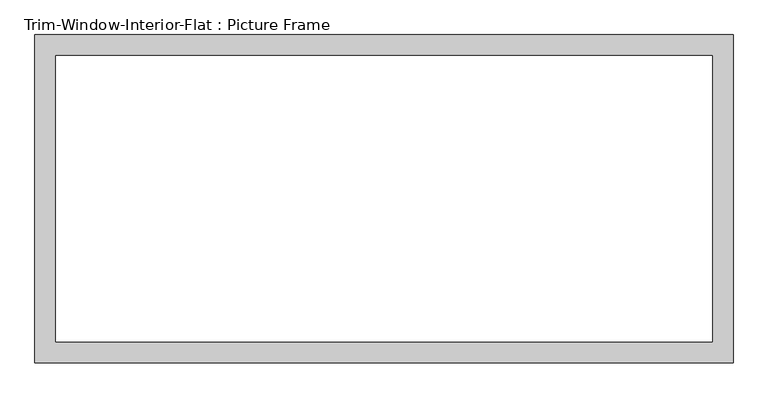
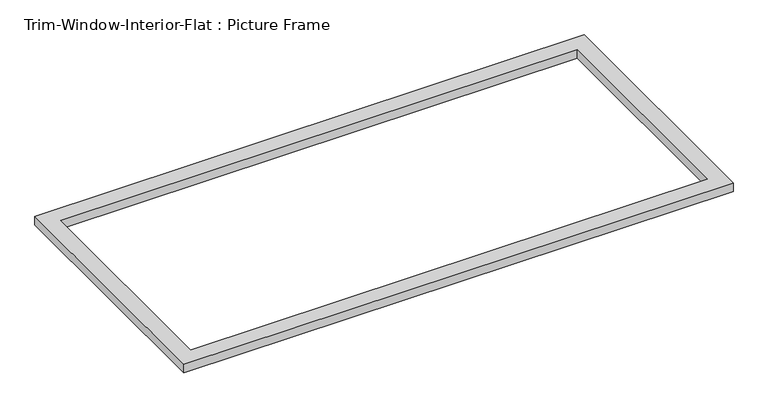
"""IFC4 building model written with IfcOpenShell, lengths in millimetres: proxy geometry, Trim-Window-Interior-Flat : Picture Frame."""

from ifc_helpers import new_model, si_unit, origin, origin_with_axes, place, context, project, spatial, polyline, outline, extrude, source, transform, mapped, element, save


def trim_window_interior_flat_picture_frame_687edbe0(model_context):
    return source(origin(), model_context, "Body", "SweptSolid", [
        extrude(outline(polyline([(958.85, -44.45), (-958.85, -44.45), (-958.85, 857.25), (958.85, 857.25), (958.85, -44.45)]), holes=[polyline([(901.7, 12.7), (901.7, 800.1), (-901.7, 800.1), (-901.7, 12.7), (901.7, 12.7)])]), origin_with_axes(), (0.0, 0.0, 1.0), 31.75),
    ])


if __name__ == "__main__":
    model = new_model("IFC4")
    model_context = context("Model", 3, world=origin())
    ifc_project = project(units=[si_unit("LENGTHUNIT", "METRE", prefix="MILLI")], contexts=[model_context])
    site = spatial("IfcSite", under=ifc_project)
    building = spatial("IfcBuilding", under=site)
    placement = place(None, origin())
    trim_window_interior_flat_picture_frame_shape = trim_window_interior_flat_picture_frame_687edbe0(model_context)
    element("IfcBuildingElementProxy", 1, Name="Trim-Window-Interior-Flat : Picture Frame", ObjectType="Trim-Window-Interior-Flat : Picture Frame", at=placement, inside=building, context=model_context, shape_type="MappedRepresentation", body=[
        mapped(trim_window_interior_flat_picture_frame_shape, transform((0.0, 0.0, 0.0), x_axis=(1.0, 0.0, 0.0), y_axis=(0.0, 1.0, 0.0), z_axis=(0.0, 0.0, 1.0))),
    ])
    save(model, "model.ifc")

# Revit data of these elements
# Type "Trim-Window-Interior-Flat : Picture Frame"
#   Trim Thickness_Picture Frame = 0.104167 ft
#   Trim Width = 0.1875 ft
#   Trim Thickness_with Sill = 0.0625 ft
#   Sill Thickness = 0.104167 ft
#   Opening Width [instance default] = 2 ft
#   Opening Height [instance default] = 3 ft
#   Default Elevation = 4 ft
#   Sill = no
#   Picture Frame = yes
#   Trim Material [instance default] = none
# Element 1 (IfcBuildingElementProxy, "Trim-Window-Interior-Flat : Picture Frame")
#   Opening Width = 6 ft
#   Opening Height = 2.666667 ft
#   Trim Material = Wood - Stained
#   Materials on its faces: "Wood - Stained"
# Materials
#   "Wood - Stained": class "Wood", colour RGB 224 178 126, transparency 0, Cost = 0
